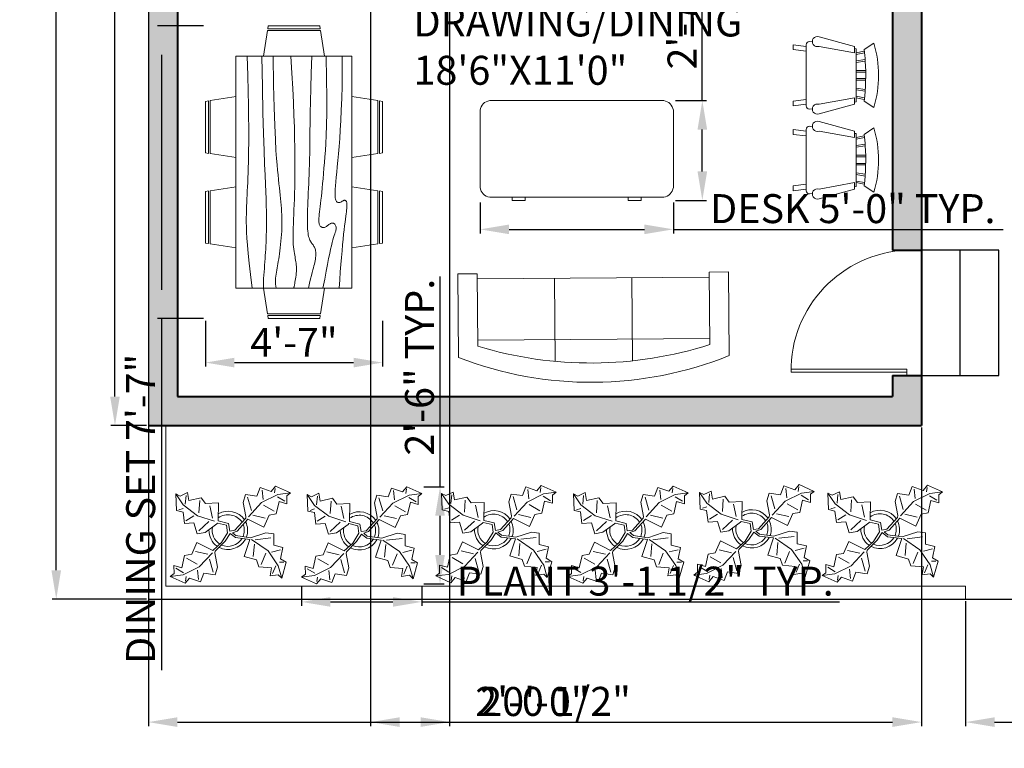
# Model space of a CAD drawing. Units: inches. Extents: x 1967493 to 1968177, y 907234 to 908105.
# Tile 1 of 5: x 1967549 to 1967854, y 907234 to 907460. Entities that reach past the tile are written whole.
import ezdxf

# ---------------------------------------------------------------- set-up
doc = ezdxf.new("R2010")
doc.units = ezdxf.units.IN
for name, color, linetype, lineweight in [('A-ANNO-DIMS', 2, 'Continuous', 18), ('A-AREA-IDEN', 7, 'Continuous', 25), ('A-DOOR', 3, 'Continuous', 20), ('A-FLOR-STRS', 7, 'Continuous', 25), ('A-FURN', 8, 'Continuous', 18), ('A-WALL', 7, 'Continuous', 40), ('C-PROP', 7, 'Continuous', 25), ('L-PLNT', 94, 'Continuous', 18)]:
    doc.layers.add(name, color=color, linetype=linetype, lineweight=lineweight)
doc.layers.add('A-WALL-PATT', color=18, linetype='Continuous', lineweight=13, true_color=0x000000)
doc.styles.get("Standard").update_dxf_attribs({"font": 'arial.ttf'})
doc.dimstyles.new('ISO-25', dxfattribs={"dimtxt": 9, "dimasz": 9, "dimexe": 1.25, "dimexo": 0.625, "dimtad": 1, "dimdec": 1, "dimrnd": 9, "dimlunit": 3, "dimtxsty": 'Standard', "dimcen": 2.5, "dimadec": 0, "dimazin": 0, "dimtfac": 1, "dimtdec": 1, "dimtmove": 0, "dimatfit": 3, "dimfxl": 1, "dimarcsym": 0})

# ---------------------------------------------------------------- blocks, each defined once
blk = doc.blocks.new('Plant - Rubber or Philodendron')
for p, q in [((8.8871, 10.7908), (9.9809, 13.4933)), ((9.9809, 13.4933), (13.3837, 12.301)), ((10.5828, 12.6946), (10.8893, 9.7953)), ((13.3837, 12.301), (14.68, 13.9039)), ((14.5816, 13.2037), (14.3848, 11.8033)), ((14.68, 13.9039), (19.3848, 11.8146)), ((-16.2005, 11.4774), (-13.9899, 8.1064)), ((-16.2005, 11.4774), (-14.8639, 10.7964)), ((-16.0159, 6.3329), (-16.2005, 11.4774)), ((-14.8639, 10.7964), (-12.6195, 11.8975)), ((-13.3174, 8.325), (-13.0735, 11.0065)), ((-12.6195, 11.8975), (-12.1909, 9.4345)), ((-12.1909, 9.4345), (-8.3829, 10.3)), ((-8.8369, 9.409), (-9.0894, 5.6095)), ((-8.3829, 10.3), (-7.0549, 8.501)), ((4.6914, 8.8812), (5.3859, 11.2828)), ((5.3859, 11.2828), (8.8871, 10.7908)), ((5.9878, 10.4842), (7.1971, 6.3869)), ((15.3859, 11.3055), (10.3916, 8.7942)), ((15.2875, 10.6053), (17.5907, 9.2105)), ((19.3848, 11.8146), (15.3859, 11.3055)), ((19.3848, 11.8146), (18.1868, 10.9119)), ((18.1868, 10.9119), (18.1925, 8.4119)), ((-14.0069, 5.8704), (-16.0159, 6.3329)), ((-15.3434, 6.5514), (-13.9984, 6.9884)), ((-13.9899, 8.1064), (-9.5434, 4.7185)), ((-7.0549, 8.501), (-3.0284, 8.6941)), ((-4.8529, 4.012), (-5.7184, 7.82)), ((-3.0284, 8.6941), (-3.0709, 3.1041)), ((4.6914, 8.8812), (5.5014, 4.4831)), ((10.3916, 8.7942), (6.2847, 4.4028)), ((14.2977, 6.1031), (10.9934, 7.9956)), ((15.7909, 9.1065), (14.8995, 5.3044)), ((18.1925, 8.4119), (15.7909, 9.1065)), ((-13.5868, 2.2894), (-14.0069, 5.8704)), ((-13.1329, 3.1804), (-10.6614, 4.727)), ((-9.5434, 4.7185), (-4.1917, 2.9888)), ((-3.0709, 3.1041), (0.0797, 2.3163)), ((2.1141, 0.2298), (5.4346, 3.9146)), ((6.1032, 3.6844), (2.8262, -0.031)), ((5.4346, 3.9146), (5.5014, 4.4831)), ((11.1089, 1.1958), (6.1032, 3.6844)), ((7.7005, 4.8881), (11.5025, 3.9967)), ((12.7005, 4.8994), (11.1089, 1.1958)), ((14.8995, 5.3044), (12.7005, 4.8994)), ((-10.6784, 2.491), (-13.5868, 2.2894)), ((-9.5858, -0.8715), (-10.6784, 2.491)), ((-9.1318, 0.0195), (-5.9793, 2.9025)), ((-7.1228, -0.443), (-3.5248, 2.2131)), ((-3.5248, 2.2131), (-3.3011, 2.4355)), ((-3.3011, 2.4355), (-0.5306, 1.7947)), ((-0.5306, 1.7947), (-0.2255, -0.5527)), ((-0.5306, 1.7947), (-0.5306, 1.7947)), ((0.0797, 2.3163), (0.4866, -0.031)), ((0.4866, -0.031), (2.1141, 0.2298)), ((-7.1228, -0.443), (-9.5858, -0.8715)), ((-2.019, -3.6148), (-0.2255, -0.5527)), ((-0.9375, -3.1608), (0.5883, -0.8135)), ((0.5883, -0.8135), (2.2447, -2.0916)), ((2.8262, -0.031), (1.3003, -0.5527)), ((1.3003, -0.5527), (2.4193, -1.4655)), ((2.2447, -2.0916), (6.7108, -2.6626)), ((2.4193, -1.4655), (6.895, -2.1175)), ((4.943, -7.9659), (6.7108, -2.6626)), ((11.6605, -0.5413), (6.895, -2.1175)), ((12.3677, -6.1981), (7.219, -2.6772)), ((8.3544, -2.7453), (13.1973, -2.1704)), ((11.6605, -0.5413), (14.1354, -0.8948)), ((14.1354, -0.8948), (14.1354, -4.4304)), ((-11.3237, -7.2629), (-9.7321, -3.5593)), ((-9.7321, -3.5593), (-4.7264, -6.0479)), ((-2.019, -3.6148), (-4.7264, -6.0479)), ((-4.0579, -6.2781), (-0.9375, -3.1608)), ((8.125, -4.0768), (7.7715, -7.9659)), ((16.2567, -5.8446), (13.4283, -6.5517)), ((14.1354, -4.4304), (16.9638, -5.1375)), ((16.9638, -5.1375), (16.2567, -8.673)), ((-14.4141, -11.4699), (-13.5228, -7.6679)), ((-13.5228, -7.6679), (-11.3237, -7.2629)), ((-12.921, -8.4665), (-9.6166, -10.359)), ((-6.3237, -7.2516), (-10.1257, -6.3602)), ((-9.0148, -11.1577), (-4.9047, -6.8122)), ((-4.611, -12.8477), (-5.8203, -8.7504)), ((-4.1246, -6.8466), (-4.0579, -6.2781)), ((-3.3146, -11.2447), (-4.1246, -6.8466)), ((8.8321, -9.0266), (4.943, -7.9659)), ((9.5392, -11.1479), (8.8321, -9.0266)), ((10.2463, -10.4408), (11.6605, -6.9053)), ((15.5496, -10.7943), (12.3677, -6.1981)), ((16.2567, -8.673), (18.0245, -9.7337)), ((-16.8157, -10.7754), (-14.4141, -11.4699)), ((-16.8101, -13.2754), (-16.8157, -10.7754)), ((-13.9107, -12.9688), (-16.2139, -11.574)), ((-14.0091, -13.669), (-9.0148, -11.1577)), ((-9.206, -15.0581), (-9.5126, -12.1588)), ((-3.3146, -11.2447), (-4.0092, -13.6463)), ((13.4283, -11.5015), (9.5392, -11.1479)), ((13.0748, -13.9763), (13.4283, -11.5015)), ((14.8425, -10.7943), (13.7819, -13.2692)), ((16.6103, -14.6834), (15.5496, -10.7943)), ((17.3174, -9.7337), (15.9032, -9.7337)), ((18.0245, -9.7337), (16.6103, -14.6834)), ((-18.008, -14.1781), (-16.8101, -13.2754)), ((-18.008, -14.1781), (-14.0091, -13.669)), ((-13.3032, -16.2674), (-18.008, -14.1781)), ((-12.0069, -14.6645), (-13.3032, -16.2674)), ((-13.2048, -15.5672), (-13.008, -14.1668)), ((-8.6042, -15.8568), (-12.0069, -14.6645)), ((-7.5103, -13.1543), (-8.6042, -15.8568)), ((-4.0092, -13.6463), (-7.5103, -13.1543)), ((15.5496, -13.6228), (13.0748, -13.9763)), ((16.6103, -14.6834), (15.5496, -13.6228))]:
    blk.add_line(p, q)
for centre, radius, start, end in [((0, 0), 6.1275, 34.37569, 120.1028), ((-0.0601, -0.2075), 5.2461, 33.82192, 124.9414), ((0.0308, 0.1664), 6, 178.6147, 235.1169), ((0.0308, 0.1664), 5, 168.1647, 238.6725), ((-0.2664, 0.1682), 5.2775, 338.4094, 20.03007), ((-0.098, 0.1364), 6.1288, 341.2017, 26.09184), ((-0.0234, 0.3825), 6.1492, 242.5812, 331.2714), ((-0.1102, 0.4886), 5.2883, 247.3711, 327.472)]:
    blk.add_arc(centre, radius, start, end)
blk = doc.blocks.new('Dining Set - 36 x 72 in.')
for p, q in [((-22.2343, 26.00059), (-23.4847, 17.99762)), ((-22.2304, 26), (-5.7608, 26)), ((-22, 27.5), (-22.1562, 26.50042)), ((-5.8416, 26.5), (-22.1534, 26.5)), ((-22, 27.5), (-6, 27.5)), ((-5.8437, 26.49966), (-6, 27.5)), ((-4.5152, 17.99762), (-5.7655, 25.99926)), ((5.7657, 26.00059), (4.5153, 17.99762)), ((5.7696, 26), (22.2392, 26)), ((6, 27.5), (5.8438, 26.50042)), ((22.1584, 26.5), (5.8466, 26.5)), ((6, 27.5), (22, 27.5)), ((22.1563, 26.49966), (22, 27.5)), ((23.4848, 17.99762), (22.2345, 25.99926)), ((36, 18), (-36, 18)), ((-36, 18), (-36, -18)), ((36, -18), (36, 18)), ((-44.0006, 8.23428), (-35.9976, 9.48474)), ((44.0006, 8.23428), (35.9976, 9.48474)), ((-45.5, 8), (-44.5004, 8.15617)), ((-45.5, 8), (-45.5, -8)), ((-44.5, -8.15843), (-44.5, 8.15338)), ((-44, 8.23041), (-44, -8.23915)), ((44, 8.23041), (44, -8.23915)), ((44.5, -8.15843), (44.5, 8.15338)), ((45.5, 8), (44.5005, 8.15617)), ((45.5, 8), (45.5, -8)), ((-44.4997, -8.15631), (-45.5, -8)), ((-35.9976, -9.48476), (-43.9993, -8.2345)), ((35.9976, -9.48476), (43.9993, -8.2345)), ((44.4997, -8.15631), (45.5, -8)), ((-36, -18), (36, -18)), ((-22.2343, -26.0006), (-23.4847, -17.99762)), ((-4.5152, -17.99762), (-5.7655, -25.99928)), ((5.7657, -26.0006), (4.5153, -17.99762)), ((23.4848, -17.99762), (22.2345, -25.99928)), ((-22.2304, -26), (-5.7608, -26)), ((-22, -27.5), (-22.1562, -26.50044)), ((-5.8416, -26.5), (-22.1534, -26.5)), ((-22, -27.5), (-6, -27.5)), ((-5.8437, -26.49967), (-6, -27.5)), ((5.7696, -26), (22.2392, -26)), ((6, -27.5), (5.8438, -26.50044)), ((22.1584, -26.5), (5.8466, -26.5)), ((6, -27.5), (22, -27.5)), ((22.1563, -26.49967), (22, -27.5))]:
    blk.add_line(p, q)
for points in [[(-36, 15), (-31.1772, 14.97754), (-26.8079, 14.91406), (-22.8538, 14.81543), (-19.276, 14.6875), (-16.0362, 14.53613), (-13.0957, 14.36718), (-10.4159, 14.18652), (-7.9583, 14), (-5.6904, 13.81315), (-3.6035, 13.63021), (-1.6954, 13.45508), (0.0365, 13.29166), (1.5945, 13.14388), (2.9811, 13.01562), (4.1988, 12.9108), (5.25, 12.83333), (6.1393, 12.78613), (6.8802, 12.76823), (7.4883, 12.77767), (7.9792, 12.8125), (8.3685, 12.87077), (8.6719, 12.95052), (8.9049, 13.0498), (9.0833, 13.16666), (9.2205, 13.29899), (9.3216, 13.44401), (9.3895, 13.59879), (9.4271, 13.76041), (9.4373, 13.92594), (9.4232, 14.09245), (9.3875, 14.257), (9.3333, 14.41666), (9.2638, 14.56917), (9.1836, 14.71484), (9.0975, 14.85465), (9.0104, 14.98958), (8.9272, 15.1206), (8.8529, 15.2487), (8.7922, 15.37483), (8.75, 15.5), (8.7305, 15.62467), (8.7344, 15.74739), (8.7617, 15.86621), (8.8125, 15.97916), (8.8867, 16.08431), (8.9844, 16.17968), (9.1055, 16.26334), (9.25, 16.33333), (9.4189, 16.38802), (9.6172, 16.42708), (9.8506, 16.45052), (10.125, 16.45833), (10.4463, 16.45052), (10.8203, 16.42708), (11.2529, 16.38802), (11.75, 16.33333), (12.3184, 16.26318), (12.9694, 16.17838), (13.7151, 16.07991), (14.5677, 15.96875), (15.5395, 15.84586), (16.6426, 15.71224), (17.8893, 15.56884), (19.2917, 15.41666), (20.859, 15.25667), (22.5879, 15.08984), (24.4721, 14.91715), (26.5052, 14.73958), (28.6809, 14.5581), (30.9929, 14.3737), (33.4347, 14.18733), (36, 14)], [(-36, 10), (-28.9766, 10.14274), (-23.1725, 10.20442), (-18.4241, 10.19775), (-14.5677, 10.13541), (-11.4399, 10.03011), (-8.877, 9.89453), (-6.7154, 9.74137), (-4.7917, 9.58333), (-2.9698, 9.43082), (-1.2246, 9.28515), (0.4415, 9.14534), (2.026, 9.01041), (3.5266, 8.87939), (4.9408, 8.7513), (6.266, 8.62516), (7.5, 8.5), (8.6411, 8.37549), (9.6914, 8.2539), (10.6538, 8.13818), (11.5312, 8.03125), (12.3267, 7.93603), (13.043, 7.85547), (13.6831, 7.79248), (14.25, 7.75), (14.7471, 7.7303), (15.1797, 7.73307), (15.5537, 7.75732), (15.875, 7.80208), (16.1494, 7.86637), (16.3828, 7.94922), (16.5811, 8.04964), (16.75, 8.16666), (16.8944, 8.29915), (17.0143, 8.44531), (17.1089, 8.60319), (17.1771, 8.77083), (17.218, 8.94629), (17.2305, 9.1276), (17.2137, 9.31282), (17.1667, 9.5), (17.0895, 9.6875), (16.987, 9.875), (16.8649, 10.0625), (16.7292, 10.25), (16.5856, 10.4375), (16.4401, 10.625), (16.2985, 10.8125), (16.1667, 11), (16.05, 11.18733), (15.9518, 11.3737), (15.8752, 11.5581), (15.8229, 11.73958), (15.798, 11.91715), (15.8034, 12.08984), (15.842, 12.25667), (15.9167, 12.41666), (16.0295, 12.56836), (16.1784, 12.70833), (16.3605, 12.83268), (16.5729, 12.9375), (16.8127, 13.01888), (17.0768, 13.07291), (17.3625, 13.0957), (17.6667, 13.08333), (17.9894, 13.03312), (18.3418, 12.94726), (18.7382, 12.82918), (19.1927, 12.68229), (19.7195, 12.51001), (20.3327, 12.31575), (21.0465, 12.10294), (21.875, 11.875), (22.8357, 11.63354), (23.959, 11.37304), (25.2786, 11.08618), (26.8282, 10.76562), (28.6414, 10.40405), (30.752, 9.99414), (33.1936, 9.52856), (36, 9)], [(-36, 5.5), (-30.7157, 5.3348), (-26.069, 5.20963), (-21.9946, 5.11767), (-18.4271, 5.05208), (-15.3009, 5.00602), (-12.5508, 4.97265), (-10.1112, 4.94515), (-7.9167, 4.91666), (-5.909, 4.88167), (-4.0586, 4.83984), (-2.3429, 4.79215), (-0.7396, 4.73958), (0.7739, 4.6831), (2.22, 4.6237), (3.6213, 4.56233), (5, 4.5), (6.373, 4.43782), (7.7344, 4.3776), (9.0723, 4.32129), (10.375, 4.27083), (11.6309, 4.22819), (12.8281, 4.19531), (13.9551, 4.17415), (15, 4.16666), (15.954, 4.17448), (16.819, 4.19791), (17.6001, 4.23698), (18.3021, 4.29166), (18.9299, 4.36198), (19.4883, 4.44791), (19.9823, 4.54948), (20.4167, 4.66666), (20.7969, 4.79899), (21.1302, 4.94401), (21.4245, 5.09879), (21.6875, 5.26041), (21.9271, 5.42594), (22.1511, 5.59245), (22.3672, 5.757), (22.5834, 5.91666), (22.8065, 6.06868), (23.0404, 6.21093), (23.2879, 6.34147), (23.5521, 6.45833), (23.8358, 6.55957), (24.142, 6.64323), (24.4735, 6.70735), (24.8334, 6.75), (25.2235, 6.76969), (25.642, 6.76692), (26.0858, 6.74267), (26.5521, 6.69791), (27.0379, 6.63362), (27.5404, 6.55078), (28.0565, 6.45036), (28.5834, 6.33333), (29.1242, 6.19987), (29.7071, 6.04687), (30.3661, 5.87044), (31.1354, 5.66666), (32.0493, 5.43164), (33.142, 5.16146), (34.4475, 4.85221), (36, 4.5)], [(-36, -1), (-30.7915, -0.6591), (-26.0195, -0.38216), (-21.6519, -0.16284), (-17.6563, 0.00521), (-14.0005, 0.12833), (-10.6523, 0.21289), (-7.5796, 0.26522), (-4.75, 0.29166), (-2.134, 0.29793), (0.2878, 0.28711), (2.5317, 0.26163), (4.6146, 0.22396), (6.5529, 0.17651), (8.3633, 0.12174), (10.0623, 0.06209), (11.6667, 0), (13.1899, -0.06201), (14.6341, -0.1211), (15.9982, -0.17432), (17.2813, -0.21875), (18.4823, -0.25147), (19.6003, -0.26953), (20.6343, -0.27002), (21.5834, -0.25), (22.4481, -0.20768), (23.2357, -0.14584), (23.9549, -0.06836), (24.6146, 0.02083), (25.2235, 0.11784), (25.7904, 0.21875), (26.3241, 0.31966), (26.8334, 0.41666), (27.3265, 0.50618), (27.8099, 0.58593), (28.2894, 0.65397), (28.7709, 0.70833), (29.2601, 0.74707), (29.763, 0.76823), (30.2855, 0.76985), (30.8334, 0.75), (31.4088, 0.70784), (31.9994, 0.64713), (32.589, 0.57275), (33.1615, 0.48958), (33.7008, 0.4025), (34.1908, 0.3164), (34.6153, 0.23616), (34.9584, 0.16666), (35.2099, 0.11165), (35.3848, 0.07031), (35.504, 0.04069), (35.5886, 0.02083), (35.6594, 0.00879), (35.7377, 0.0026), (35.8442, 0.00032), (36, 0)], [(-36, -6.5), (-27.1843, -6.31267), (-20.084, -6.1263), (-14.469, -5.9419), (-10.1094, -5.76042), (-6.7752, -5.58285), (-4.2363, -5.41016), (-2.2629, -5.24333), (-0.625, -5.08334), (0.8708, -4.93099), (2.2715, -4.78646), (3.5872, -4.64974), (4.8281, -4.52084), (6.0046, -4.39974), (7.127, -4.28646), (8.2053, -4.18099), (9.25, -4.08334), (10.2705, -3.99382), (11.2734, -3.91407), (12.2647, -3.84603), (13.25, -3.79167), (14.2354, -3.75293), (15.2266, -3.73177), (16.2295, -3.73015), (17.25, -3.75), (18.2912, -3.79248), (19.3451, -3.85547), (20.4009, -3.93604), (21.4479, -4.03125), (22.4754, -4.13819), (23.4727, -4.25391), (24.4289, -4.37549), (25.3334, -4.5), (26.1785, -4.62492), (26.9694, -4.74935), (27.7145, -4.87281), (28.4219, -4.99479), (29.1, -5.11483), (29.7572, -5.23242), (30.4016, -5.34709), (31.0417, -5.45834), (31.6837, -5.56437), (32.3262, -5.65821), (32.9658, -5.73153), (33.599, -5.77604), (34.2224, -5.78345), (34.8327, -5.74545), (35.4264, -5.65373), (36, -5.5)], [(-36, -10), (-26.4022, -9.81299), (-18.4675, -9.62891), (-11.9839, -9.45069), (-6.7396, -9.28125), (-2.5226, -9.12354), (0.8789, -8.98047), (3.6769, -8.85498), (6.0833, -8.75), (8.2767, -8.66765), (10.3021, -8.60677), (12.1712, -8.56543), (13.8958, -8.54167), (15.4876, -8.53353), (16.9583, -8.53907), (18.3197, -8.55632), (19.5834, -8.58334), (20.7616, -8.61841), (21.8685, -8.66081), (22.9188, -8.71004), (23.9271, -8.76563), (24.9081, -8.82707), (25.8763, -8.89388), (26.8465, -8.96558), (27.8334, -9.04167), (28.8474, -9.12118), (29.8828, -9.20117), (30.93, -9.27824), (31.9792, -9.34896), (33.0205, -9.40991), (34.0443, -9.45768), (35.0407, -9.48885), (36, -9.5)], [(-36, -14.5), (-30.0881, -14.33513), (-25.0332, -14.21224), (-20.7312, -14.12647), (-17.0781, -14.07292), (-13.97, -14.04671), (-11.3027, -14.04297), (-8.9724, -14.05681), (-6.875, -14.08334), (-4.9224, -14.11833), (-3.0905, -14.16016), (-1.3709, -14.20785), (0.2448, -14.26042), (1.7647, -14.3169), (3.1973, -14.3763), (4.5507, -14.43767), (5.8333, -14.5), (7.0554, -14.5621), (8.235, -14.62175), (9.3922, -14.67652), (10.5469, -14.72396), (11.7192, -14.76164), (12.929, -14.78711), (14.1965, -14.79794), (15.5417, -14.79167), (16.9933, -14.76424), (18.6152, -14.70508), (20.4804, -14.60197), (22.6615, -14.44271), (25.2312, -14.21509), (28.2624, -13.9069), (31.8277, -13.50594), (36, -13)]]:
    blk.add_lwpolyline(points)
blk = doc.blocks.new('Sofa - Roundback 7 ft.')
for p, q in [((-12.00002, -32.4421), (-12.00003, -6.5971)), ((11.99997, -32.4421), (11.99998, -6.5971)), ((-36.000027, -34), (-36.000027, -11.4696)), ((35.99998, -34), (35.99998, -11.4696)), ((-35.999844, -13.3819), (35.9998, -13.3819)), ((-36.000027, -32.4421), (35.99998, -32.4421))]:
    blk.add_line(p, q)
for points in [[(-36.000027, -34), (-42.000027, -34), (-42.000027, -8)], [(41.99998, -8), (41.99998, -34), (35.99998, -34)]]:
    blk.add_lwpolyline(points)
for centre, radius, start, end in [((0, -114.25), 114.25, 68.43141, 111.5686), ((-0.00001, -127.1968), 121.1968, 72.72033, 107.2797)]:
    blk.add_arc(centre, radius, start, end)
blk = doc.blocks.new('Desk - 30 x 60 in.')
for p, q in [((-26.999995, 0), (26.999995, 0)), ((-29.999995, -27), (-29.999995, -3)), ((29.999995, -3), (29.999995, -27)), ((26.999995, -30), (-26.999995, -30)), ((-20.000005, -30), (-20.000005, -31)), ((-16.000005, -31), (-16.000005, -30)), ((15.999995, -31), (15.999995, -30)), ((19.999995, -30), (19.999995, -31)), ((-20.000005, -31), (-16.000005, -31)), ((19.999995, -31), (15.999995, -31))]:
    blk.add_line(p, q)
for centre, start, end in [((-26.499995, -3.5), 98.1301, 171.8699), ((26.499995, -3.5), 8.130102, 81.8699), ((-26.499995, -26.5), 188.1301, 261.8699), ((26.499995, -26.5), 278.1301, 351.8699)]:
    blk.add_arc(centre, 3.535534, start, end)
blk = doc.blocks.new('Chair - Rocking')
for p, q in [((-8, -4.5), (-10, -1.5)), ((8, -4.5), (10, -1.5)), ((-7.5, -4.5), (-7, -7)), ((-6.5, -7), (-7.02225, -4.43)), ((-4.5, -7), (-4.96674, -4.19951)), ((-4, -7), (-4.40532, -4.16272)), ((-1.5, -4.05012), (-1.5, -7)), ((-1, -7), (-1, -4.05012)), ((1, -7), (1, -4.04655)), ((1.5, -4.05012), (1.5, -7)), ((4, -7), (4.40187, -4.18694)), ((4.5, -7), (4.96761, -4.19437)), ((6.5, -7), (7, -4.4057)), ((7.5, -4.5), (7, -7)), ((-9, -7.5), (-12, -18.49999)), ((-7, -7.5), (-9, -7.5)), ((-9, -18.49999), (-7, -7.5)), ((-8.23428, -6.99939), (-8.3093, -7.47958)), ((-8.23041, -7), (8.23915, -7)), ((7, -7.5), (9, -7.5)), ((9, -18.49999), (7, -7.5)), ((8.31071, -7.48854), (8.23449, -7.00073)), ((9, -7.5), (12, -18.49999)), ((-10.36644, -20.64523), (-10.5, -21.49999)), ((10.5, -21.49999), (10.3575, -20.58798)), ((-9, -22.49999), (-9.5, -26.49999)), ((0, -22.49999), (-9.5, -22.49999)), ((-8, -26.49999), (-7.5, -22.49999)), ((0, -22.49999), (9.5, -22.49999)), ((8, -26.49999), (7.5, -22.49999)), ((9, -22.49999), (9.5, -26.49999)), ((-9.5, -26.49999), (-8, -26.49999)), ((9.5, -26.49999), (8, -26.49999))]:
    blk.add_line(p, q)
for centre, radius, start, end in [((0, -34.08333), 34.08333, 72.93847, 107.0615), ((0, -68.25004), 64.25, 93.92211, 97.15267), ((0, -68.25004), 64.25, 82.84733, 93.92211), ((-10.5, -18.99999), 1.58114, 161.5651, 18.43495), ((10.5, -18.99999), 1.58114, 161.5651, 18.43495), ((-9.5, -21.49999), 1, 180, 270), ((9.5, -21.49999), 1, 270, 0)]:
    blk.add_arc(centre, radius, start, end)
blk = doc.blocks.new('*D12')
at = {"layer": 'A-ANNO-DIMS', "color": 0, "lineweight": -2, "transparency": 16777216}
for p, q in [((1967588.15, 908000.17), (1967558.93, 908000.17)), ((1967560.18, 907289.17), (1967560.18, 907991.17)), ((1967588.15, 907280.17), (1967558.93, 907280.17))]:
    blk.add_line(p, q, dxfattribs=at)
at = {"layer": 'A-ANNO-DIMS', "color": 0, "transparency": 16777216}
for points in [[(1967558.68, 907991.17), (1967561.68, 907991.17), (1967560.18, 908000.17)], [(1967558.68, 907289.17), (1967561.68, 907289.17), (1967560.18, 907280.17)]]:
    blk.add_solid(points, dxfattribs=at)
at = {"layer": 'Defpoints', "color": 0, "transparency": 16777216}
for p in [(1967560.18, 908000.17), (1967588.78, 908000.17), (1967588.78, 907280.17)]:
    blk.add_point(p, dxfattribs=at)
at = {"layer": 'A-ANNO-DIMS', "color": 0, "transparency": 16777216, "insert": (1967554.96, 907640.17), "char_height": 9, "attachment_point": 5, "rotation": 90}
blk.add_mtext("60'", dxfattribs=at)
blk = doc.blocks.new('*D13')
at = {"layer": 'A-ANNO-DIMS', "color": 0, "lineweight": -2, "transparency": 16777216}
for p, q in [((1967588.15, 908000.17), (1967577.16, 908000.17)), ((1967578.41, 907343.17), (1967578.41, 907991.17)), ((1967588.15, 907334.17), (1967577.16, 907334.17))]:
    blk.add_line(p, q, dxfattribs=at)
at = {"layer": 'A-ANNO-DIMS', "color": 0, "transparency": 16777216}
for points in [[(1967576.91, 907991.17), (1967579.91, 907991.17), (1967578.41, 908000.17)], [(1967576.91, 907343.17), (1967579.91, 907343.17), (1967578.41, 907334.17)]]:
    blk.add_solid(points, dxfattribs=at)
at = {"layer": 'Defpoints', "color": 0, "transparency": 16777216}
for p in [(1967578.41, 908000.17), (1967588.78, 908000.17), (1967588.78, 907334.17)]:
    blk.add_point(p, dxfattribs=at)
at = {"layer": 'A-ANNO-DIMS', "color": 0, "transparency": 16777216, "insert": (1967573.19, 907667.17), "char_height": 9, "attachment_point": 5, "rotation": 90}
blk.add_mtext('55\'-6"', dxfattribs=at)
blk = doc.blocks.new('*D20')
at = {"layer": 'A-ANNO-DIMS', "color": 0, "lineweight": -2, "transparency": 16777216}
for p, q in [((1967636.31, 907284.35), (1967636.31, 907278.11)), ((1967673.71, 907284.35), (1967673.71, 907278.11)), ((1967645.31, 907279.36), (1967664.71, 907279.36)), ((1967673.71, 907279.36), (1967803.36, 907279.36))]:
    blk.add_line(p, q, dxfattribs=at)
at = {"layer": 'A-ANNO-DIMS', "color": 0, "transparency": 16777216}
for points in [[(1967645.31, 907280.86), (1967645.31, 907277.86), (1967636.31, 907279.36)], [(1967664.71, 907280.86), (1967664.71, 907277.86), (1967673.71, 907279.36)]]:
    blk.add_solid(points, dxfattribs=at)
at = {"layer": 'Defpoints', "color": 0, "transparency": 16777216}
for p in [(1967636.31, 907284.97), (1967673.71, 907284.97), (1967673.71, 907279.36)]:
    blk.add_point(p, dxfattribs=at)
at = {"layer": 'A-ANNO-DIMS', "color": 0, "transparency": 16777216, "insert": (1967743.03, 907284.65), "char_height": 9, "attachment_point": 5}
blk.add_mtext('PLANT 3\'-1 1/2" TYP.', dxfattribs=at)
blk = doc.blocks.new('*D21')
at = {"layer": 'A-ANNO-DIMS', "color": 0, "lineweight": -2, "transparency": 16777216}
for p, q in [((1967679.32, 907315.14), (1967679.32, 907380.41)), ((1967674.33, 907315.14), (1967680.57, 907315.14)), ((1967679.32, 907293.97), (1967679.32, 907306.14)), ((1967674.33, 907284.97), (1967680.57, 907284.97))]:
    blk.add_line(p, q, dxfattribs=at)
at = {"layer": 'A-ANNO-DIMS', "color": 0, "transparency": 16777216}
for points in [[(1967677.82, 907306.14), (1967680.82, 907306.14), (1967679.32, 907315.14)], [(1967677.82, 907293.97), (1967680.82, 907293.97), (1967679.32, 907284.97)]]:
    blk.add_solid(points, dxfattribs=at)
at = {"layer": 'Defpoints', "color": 0, "transparency": 16777216}
for p in [(1967673.71, 907315.14), (1967679.32, 907315.14), (1967673.71, 907284.97)]:
    blk.add_point(p, dxfattribs=at)
at = {"layer": 'A-ANNO-DIMS', "color": 0, "transparency": 16777216, "insert": (1967674.1, 907352.28), "char_height": 9, "attachment_point": 5, "rotation": 90}
blk.add_mtext('2\'-6" TYP.', dxfattribs=at)
blk = doc.blocks.new('*D32')
at = {"layer": 'A-ANNO-DIMS', "color": 0, "lineweight": -2, "transparency": 16777216}
for p, q in [((1967691.75, 907403.47), (1967691.75, 907393.85)), ((1967751.75, 907403.47), (1967751.75, 907393.85)), ((1967700.75, 907395.1), (1967742.75, 907395.1)), ((1967751.75, 907395.1), (1967854.15, 907395.1))]:
    blk.add_line(p, q, dxfattribs=at)
at = {"layer": 'A-ANNO-DIMS', "color": 0, "transparency": 16777216}
for points in [[(1967700.75, 907396.6), (1967700.75, 907393.6), (1967691.75, 907395.1)], [(1967742.75, 907396.6), (1967742.75, 907393.6), (1967751.75, 907395.1)]]:
    blk.add_solid(points, dxfattribs=at)
at = {"layer": 'Defpoints', "color": 0, "transparency": 16777216}
for p in [(1967691.75, 907404.1), (1967751.75, 907404.1), (1967751.75, 907395.1)]:
    blk.add_point(p, dxfattribs=at)
at = {"layer": 'A-ANNO-DIMS', "color": 0, "transparency": 16777216, "insert": (1967807.45, 907400.37), "char_height": 9, "attachment_point": 5}
blk.add_mtext('DESK 5\'-0" TYP.', dxfattribs=at)
blk = doc.blocks.new('*D33')
at = {"layer": 'A-ANNO-DIMS', "color": 0, "lineweight": -2, "transparency": 16777216}
for p, q in [((1967760.75, 907435.1), (1967760.75, 907500.36)), ((1967752.38, 907435.1), (1967762, 907435.1)), ((1967760.75, 907413.1), (1967760.75, 907426.1)), ((1967752.38, 907404.1), (1967762, 907404.1))]:
    blk.add_line(p, q, dxfattribs=at)
at = {"layer": 'A-ANNO-DIMS', "color": 0, "transparency": 16777216}
for points in [[(1967759.25, 907426.1), (1967762.25, 907426.1), (1967760.75, 907435.1)], [(1967759.25, 907413.1), (1967762.25, 907413.1), (1967760.75, 907404.1)]]:
    blk.add_solid(points, dxfattribs=at)
at = {"layer": 'Defpoints', "color": 0, "transparency": 16777216}
for p in [(1967751.75, 907435.1), (1967760.75, 907435.1), (1967751.75, 907404.1)]:
    blk.add_point(p, dxfattribs=at)
at = {"layer": 'A-ANNO-DIMS', "color": 0, "transparency": 16777216, "insert": (1967755.61, 907472.23), "char_height": 9, "attachment_point": 5, "rotation": 90}
blk.add_mtext('2\'-7" TYP.', dxfattribs=at)
blk = doc.blocks.new('*D38')
at = {"layer": 'A-ANNO-DIMS', "color": 0, "lineweight": -2, "transparency": 16777216}
for p, q in [((1967605.85, 907458.36), (1967591.58, 907458.36)), ((1967592.83, 907449.36), (1967592.83, 907376.36)), ((1967605.85, 907367.36), (1967591.58, 907367.36)), ((1967592.83, 907367.36), (1967592.83, 907258.19))]:
    blk.add_line(p, q, dxfattribs=at)
at = {"layer": 'A-ANNO-DIMS', "color": 0, "transparency": 16777216}
for points in [[(1967591.33, 907449.36), (1967594.33, 907449.36), (1967592.83, 907458.36)], [(1967591.33, 907376.36), (1967594.33, 907376.36), (1967592.83, 907367.36)]]:
    blk.add_solid(points, dxfattribs=at)
at = {"layer": 'Defpoints', "color": 0, "transparency": 16777216}
for p in [(1967606.48, 907458.36), (1967592.83, 907367.36), (1967606.48, 907367.36)]:
    blk.add_point(p, dxfattribs=at)
at = {"layer": 'A-ANNO-DIMS', "color": 0, "transparency": 16777216, "insert": (1967587.55, 907308.27), "char_height": 9, "attachment_point": 5, "rotation": 90}
blk.add_mtext('DINING SET 7\'-7"', dxfattribs=at)
blk = doc.blocks.new('*D39')
at = {"layer": 'A-ANNO-DIMS', "color": 0, "lineweight": -2, "transparency": 16777216}
for p, q in [((1967606.48, 907366.73), (1967606.48, 907352.46)), ((1967661.48, 907366.73), (1967661.48, 907352.46)), ((1967615.48, 907353.71), (1967652.48, 907353.71))]:
    blk.add_line(p, q, dxfattribs=at)
at = {"layer": 'A-ANNO-DIMS', "color": 0, "transparency": 16777216}
for points in [[(1967615.48, 907355.21), (1967615.48, 907352.21), (1967606.48, 907353.71)], [(1967652.48, 907355.21), (1967652.48, 907352.21), (1967661.48, 907353.71)]]:
    blk.add_solid(points, dxfattribs=at)
at = {"layer": 'Defpoints', "color": 0, "transparency": 16777216}
for p in [(1967606.48, 907367.36), (1967661.48, 907367.36), (1967661.48, 907353.71)]:
    blk.add_point(p, dxfattribs=at)
at = {"layer": 'A-ANNO-DIMS', "color": 0, "transparency": 16777216, "insert": (1967633.98, 907358.83), "char_height": 9, "attachment_point": 5}
blk.add_mtext('4\'-7"', dxfattribs=at)
blk = doc.blocks.new('*D46')
at = {"layer": 'A-ANNO-DIMS', "color": 0, "lineweight": -2, "transparency": 16777216}
for p, q in [((1967842.47, 907279.54), (1967842.47, 907240.77)), ((1968059.78, 907279.54), (1968059.78, 907240.77)), ((1967851.47, 907242.02), (1968050.78, 907242.02))]:
    blk.add_line(p, q, dxfattribs=at)
at = {"layer": 'A-ANNO-DIMS', "color": 0, "transparency": 16777216}
for points in [[(1967851.47, 907243.52), (1967851.47, 907240.52), (1967842.47, 907242.02)], [(1968050.78, 907243.52), (1968050.78, 907240.52), (1968059.78, 907242.02)]]:
    blk.add_solid(points, dxfattribs=at)
at = {"layer": 'Defpoints', "color": 0, "transparency": 16777216}
for p in [(1967842.47, 907280.17), (1968059.78, 907280.17), (1968059.78, 907242.02)]:
    blk.add_point(p, dxfattribs=at)
at = {"layer": 'A-ANNO-DIMS', "color": 0, "transparency": 16777216, "insert": (1967951.12, 907247.29), "char_height": 9, "attachment_point": 5}
blk.add_mtext('18\'-1 1/2"', dxfattribs=at)
blk = doc.blocks.new('*D47')
at = {"layer": 'A-ANNO-DIMS', "color": 0, "lineweight": -2, "transparency": 16777216}
for p, q in [((1967588.78, 907333.54), (1967588.78, 907240.77)), ((1967828.78, 907333.54), (1967828.78, 907240.77)), ((1967597.78, 907242.02), (1967819.78, 907242.02))]:
    blk.add_line(p, q, dxfattribs=at)
at = {"layer": 'A-ANNO-DIMS', "color": 0, "transparency": 16777216}
for points in [[(1967597.78, 907243.52), (1967597.78, 907240.52), (1967588.78, 907242.02)], [(1967819.78, 907243.52), (1967819.78, 907240.52), (1967828.78, 907242.02)]]:
    blk.add_solid(points, dxfattribs=at)
at = {"layer": 'Defpoints', "color": 0, "transparency": 16777216}
for p in [(1967588.78, 907334.17), (1967828.78, 907334.17), (1967828.78, 907242.02)]:
    blk.add_point(p, dxfattribs=at)
at = {"layer": 'A-ANNO-DIMS', "color": 0, "transparency": 16777216, "insert": (1967708.78, 907247.24), "char_height": 9, "attachment_point": 5}
blk.add_mtext('20\'-0"', dxfattribs=at)
blk = doc.blocks.new('*D52')
at = {"layer": 'A-ANNO-DIMS', "color": 0, "lineweight": -2, "transparency": 16777216}
for p, q in [((1967657.78, 907720.78), (1967657.78, 907240.77)), ((1967682.26, 907720.78), (1967682.26, 907240.77)), ((1967666.78, 907242.02), (1967673.26, 907242.02)), ((1967682.26, 907242.02), (1967737.56, 907242.02))]:
    blk.add_line(p, q, dxfattribs=at)
at = {"layer": 'A-ANNO-DIMS', "color": 0, "transparency": 16777216}
for points in [[(1967666.78, 907243.52), (1967666.78, 907240.52), (1967657.78, 907242.02)], [(1967673.26, 907243.52), (1967673.26, 907240.52), (1967682.26, 907242.02)]]:
    blk.add_solid(points, dxfattribs=at)
at = {"layer": 'Defpoints', "color": 0, "transparency": 16777216}
for p in [(1967657.78, 907721.4), (1967682.26, 907721.4), (1967682.26, 907242.02)]:
    blk.add_point(p, dxfattribs=at)
at = {"layer": 'A-ANNO-DIMS', "color": 0, "transparency": 16777216, "insert": (1967714.41, 907247.29), "char_height": 9, "attachment_point": 5}
blk.add_mtext('2\'-0 1/2"', dxfattribs=at)

msp = doc.modelspace()

# ---------------------------------------------------------------- hatches: boundary and pattern name
at = {"layer": 'A-WALL-PATT'}
h = msp.add_hatch(color=256, dxfattribs=at)
h.dxf.hatch_style = 1
h.paths.add_polyline_path([(1967597.78, 907991.17), (1967717.78, 907991.17), (1967717.78, 907980.85), (1967726.78, 907980.85), (1967726.78, 907991.17), (1967885.78, 907991.17), (1967885.78, 907978.94), (1967894.78, 907978.94), (1967894.78, 907991.17), (1968059.78, 907991.17), (1968059.78, 907943.17), (1968039.39, 907943.17), (1968039.39, 907934.17), (1968059.78, 907934.17), (1968059.78, 907790.17), (1968052.82, 907790.17), (1968052.82, 907781.17), (1968059.78, 907781.17), (1968059.78, 907635.17), (1968052.82, 907635.17), (1968052.82, 907626.17), (1968059.78, 907626.17), (1968059.78, 907532.17), (1967892.06, 907532.17), (1967892.06, 907523.17), (1967951.97, 907523.17), (1967951.97, 907525.77), (1968004.23, 907525.77), (1968004.23, 907523.17), (1968059.78, 907523.17), (1968059.78, 907280.17), (1968068.78, 907280.17), (1968068.78, 908000.17), (1967588.78, 908000.17), (1967588.78, 907334.17), (1967828.78, 907334.17), (1967828.78, 907349.71), (1967819.78, 907349.71), (1967819.78, 907343.17), (1967597.78, 907343.17), (1967597.78, 907475.17), (1967774.78, 907475.17), (1967774.78, 907487.51), (1967765.78, 907487.51), (1967765.78, 907479.67), (1967597.78, 907479.67), (1967597.78, 907527.67), (1967604.66, 907527.67), (1967604.66, 907532.17), (1967597.78, 907532.17), (1967597.78, 907790.17), (1967597.78, 907934.17), (1967607.68, 907934.17), (1967607.68, 907943.17), (1967597.78, 907943.17)])
h.paths.add_polyline_path([(1967726.78, 907956.85), (1967717.78, 907956.85), (1967717.78, 907943.17), (1967726.78, 907943.17)], flags=17)
h.paths.add_polyline_path([(1967731.77, 907943.17), (1967651.01, 907943.17), (1967639.17, 907943.17), (1967639.17, 907934.17), (1967651.01, 907934.17), (1967731.77, 907934.17)], flags=17)
h.paths.add_polyline_path([(1967810.78, 907895.17), (1967774.78, 907895.17), (1967774.78, 907903.7), (1967765.78, 907903.7), (1967765.78, 907849.82), (1967765.78, 907834.76), (1967774.78, 907834.76), (1967774.78, 907849.82), (1967774.78, 907886.17), (1967810.78, 907886.17)], flags=17)
h.paths.add_polyline_path([(1967855.78, 907903.7), (1967846.78, 907903.7), (1967846.78, 907895.17), (1967845.59, 907895.17), (1967845.59, 907886.17), (1967846.78, 907886.17), (1967846.78, 907849.82), (1967846.78, 907834.76), (1967855.78, 907834.76), (1967855.78, 907849.82)], flags=17)
h.paths.add_polyline_path([(1968003.67, 907943.17), (1967999.78, 907943.17), (1967999.78, 907946.67), (1967990.78, 907946.67), (1967990.78, 907943.17), (1967881.11, 907943.17), (1967881.11, 907934.17), (1968003.67, 907934.17)], flags=17)
h.paths.add_polyline_path([(1967999.78, 907991.17), (1967990.78, 907991.17), (1967990.78, 907969.75, -0.052013), (1967995.28, 907969.73), (1967999.78, 907969.73)], flags=17)
h.paths.add_polyline_path([(1967777.59, 907790.17), (1967774.78, 907790.17), (1967774.78, 907796.26), (1967765.78, 907796.26), (1967765.78, 907790.17), (1967648.78, 907790.17), (1967648.78, 907769.17), (1967597.78, 907769.17), (1967597.78, 907760.17), (1967648.78, 907760.17), (1967648.78, 907749.33), (1967657.78, 907749.33), (1967657.78, 907781.17), (1967765.78, 907781.17), (1967765.78, 907721), (1967774.78, 907721), (1967774.78, 907781.17), (1967777.59, 907781.17)], flags=17)
h.paths.add_polyline_path([(1968016.82, 907790.17), (1967855.78, 907790.17), (1967855.78, 907796.26), (1967846.78, 907796.26), (1967846.78, 907790.17), (1967843.5, 907790.17), (1967843.5, 907781.17), (1967855.78, 907781.17), (1968002.78, 907781.17), (1968002.78, 907767.09), (1968011.78, 907767.09), (1968011.78, 907781.17), (1968016.82, 907781.17)], flags=17)
h.paths.add_polyline_path([(1968011.78, 907731.09), (1968002.78, 907731.09), (1968002.78, 907698.5), (1968011.78, 907698.5)], flags=17)
h.paths.add_polyline_path([(1968011.78, 907662.5), (1968002.78, 907662.5), (1968002.78, 907635.17), (1967892.06, 907635.17), (1967892.06, 907626.17), (1968016.82, 907626.17), (1968016.82, 907635.17), (1968011.78, 907635.17)], flags=17)
h.paths.add_polyline_path([(1967774.78, 907679.04), (1967765.78, 907679.04), (1967765.78, 907673.17), (1967657.78, 907673.17), (1967657.78, 907679.08), (1967648.78, 907679.08), (1967648.78, 907673.17), (1967639.33, 907673.17), (1967639.33, 907664.17), (1967765.78, 907664.17), (1967765.78, 907577.1), (1967768.96, 907577.1, -0.009361), (1967770.28, 907577.1), (1967774.78, 907577.1), (1967774.78, 907626.17), (1967779.99, 907626.17), (1967779.99, 907635.17), (1967774.78, 907635.17)], flags=17)
h.paths.add_polyline_path([(1967603.33, 907673.17), (1967597.78, 907673.17), (1967597.78, 907664.17), (1967603.33, 907664.17)], flags=17)
h.paths.add_polyline_path([(1967774.78, 907540.27), (1967765.78, 907540.27), (1967765.78, 907532.17), (1967644.82, 907532.17), (1967644.82, 907527.67), (1967765.78, 907527.67), (1967765.78, 907522.83), (1967774.78, 907522.83)], flags=17)
h.paths.add_polyline_path([(1967828.78, 907475.17), (1967828.78, 907479.67), (1967828.78, 907523.17), (1967834.39, 907523.17), (1967834.39, 907532.17), (1967828.78, 907532.17), (1967813.83, 907532.17), (1967813.83, 907527.67), (1967819.78, 907527.67), (1967819.78, 907479.67), (1967819.78, 907475.17), (1967819.78, 907388.61), (1967828.78, 907388.61)], flags=17)

# ---------------------------------------------------------------- linework, layer by layer
at = {"layer": 'A-DOOR'}
for p, q in [((1967788.28, 907350.71), (1967788.28, 907351.71)), ((1967788.28, 907351.71), (1967824.28, 907351.71)), ((1967824.28, 907351.71), (1967824.28, 907350.71)), ((1967824.28, 907350.71), (1967788.28, 907350.71)), ((1967824.28, 907349.71), (1967824.28, 907350.71))]:
    msp.add_line(p, q, dxfattribs=at)
msp.add_arc((1967825.71, 907351.21), 37.43, 92.1838, 180.7654, dxfattribs=at)
at = {"layer": 'A-FLOR-STRS'}
for p, q in [((1967852.78, 907388.61), (1967828.78, 907388.61)), ((1967840.78, 907349.71), (1967840.78, 907388.61)), ((1967852.78, 907349.71), (1967852.78, 907388.61)), ((1967828.78, 907349.71), (1967852.78, 907349.71))]:
    msp.add_line(p, q, dxfattribs=at)
at = {"layer": 'A-WALL'}
for p, q in [((1967597.78, 907475.17), (1967597.78, 907343.17)), ((1967819.78, 907475.17), (1967819.78, 907388.61)), ((1967828.78, 907475.17), (1967828.78, 907334.17)), ((1967819.78, 907388.61), (1967828.78, 907388.61)), ((1967819.78, 907349.71), (1967828.78, 907349.71)), ((1967819.78, 907349.71), (1967819.78, 907343.17)), ((1967597.78, 907343.17), (1967819.78, 907343.17)), ((1967588.78, 907334.17), (1967828.78, 907334.17))]:
    msp.add_line(p, q, dxfattribs=at)
at = {"layer": 'C-PROP'}
for p, q in [((1967588.78, 908000.17), (1967588.78, 907280.17)), ((1967588.78, 907280.17), (1968068.78, 907280.17))]:
    msp.add_line(p, q, dxfattribs=at)
at = {"layer": 'L-PLNT'}
for p, q in [((1967594.25, 907334.17), (1967594.25, 907284.24)), ((1967594.25, 907284.24), (1967842.47, 907284.24)), ((1967842.47, 907284.24), (1967842.47, 907280.17))]:
    msp.add_line(p, q, dxfattribs=at)

# ---------------------------------------------------------------- block references
at = {"layer": 'A-FURN'}
for name, p, rotation in [('Dining Set - 36 x 72 in.', (1967633.98, 907412.86), 270), ('Chair - Rocking', (1967815.48, 907442.95), 270), ('Chair - Rocking', (1967815.48, 907416.61), 270), ('Sofa - Roundback 7 ft.', (1967727.14, 907347.58), 180.4199088596836)]:
    msp.add_blockref(name, p, dxfattribs=dict(at, rotation=rotation))
msp.add_blockref('Desk - 30 x 60 in.', (1967721.75, 907435.1), dxfattribs=at)
at = {"layer": 'L-PLNT'}
for p in [(1967613.55, 907301.41), (1967654.32, 907301.24), (1967696.01, 907301.59), (1967736.98, 907301.43), (1967776.1, 907301.88), (1967815.94, 907301.71)]:
    msp.add_blockref('Plant - Rubber or Philodendron', p, dxfattribs=at)

# ---------------------------------------------------------------- texts
at = {"layer": 'A-AREA-IDEN', "insert": (1967671.08, 907464.02), "char_height": 9, "attachment_point": 1}
msp.add_mtext_dynamic_manual_height_columns('DRAWING/DINING\\P18\'6"X11\'0"', width=158.9597, gutter_width=12.5, heights=[0], dxfattribs=at)

# ---------------------------------------------------------------- dimensions: what is measured, and where the dimension line sits
at = {"layer": 'A-ANNO-DIMS'}
for base, p1, picture, middle in [((1967560.18, 908000.17), (1967588.78, 907280.17), '*D12', (1967554.96, 907640.17)), ((1967578.41, 908000.17), (1967588.78, 907334.17), '*D13', (1967573.19, 907667.17))]:
    dim = msp.add_linear_dim(base=base, p1=p1, p2=(1967588.78, 908000.17), angle=90, dimstyle='ISO-25', override={"dimclrd": 0, "dimclre": 0, "dimclrt": 0}, dxfattribs=at)
    dim.commit()
    dim.dimension.update_dxf_attribs({"geometry": picture, "text_midpoint": middle})
for base, p1, p2, picture, middle in [((1967682.26, 907242.02), (1967657.78, 907721.4), (1967682.26, 907721.4), '*D52', (1967714.41, 907247.29)), ((1967661.48, 907353.71), (1967606.48, 907367.36), (1967661.48, 907367.36), '*D39', (1967633.98, 907358.83)), ((1967828.78, 907242.02), (1967588.78, 907334.17), (1967828.78, 907334.17), '*D47', (1967708.78, 907247.24)), ((1968059.78, 907242.02), (1967842.47, 907280.17), (1968059.78, 907280.17), '*D46', (1967951.12, 907247.29))]:
    dim = msp.add_linear_dim(base=base, p1=p1, p2=p2, dimstyle='ISO-25', override={"dimdec": 1, "dimlfac": 1, "dimrnd": 0, "dimzin": 1, "dimdsep": 46, "dimlunit": 4, "dimfrac": 2}, dxfattribs=at)
    dim.commit()
    dim.dimension.update_dxf_attribs({"geometry": picture, "text_midpoint": middle})
for base, p1, p2, angle, text, picture, middle in [((1967760.75, 907435.1), (1967751.75, 907404.1), (1967751.75, 907435.1), 90, '<> TYP.', '*D33', (1967755.61, 907472.23)), ((1967592.83, 907367.36), (1967606.48, 907458.36), (1967606.48, 907367.36), 270, 'DINING SET <>', '*D38', (1967587.55, 907308.27)), ((1967679.32, 907315.14), (1967673.71, 907284.97), (1967673.71, 907315.14), 90, '<> TYP.', '*D21', (1967674.1, 907352.28))]:
    dim = msp.add_linear_dim(base=base, p1=p1, p2=p2, angle=angle, text=text, dimstyle='ISO-25', override={"dimdec": 1, "dimlfac": 1, "dimrnd": 0, "dimzin": 1, "dimdsep": 46, "dimlunit": 4, "dimfrac": 2}, dxfattribs=at)
    dim.commit()
    dim.dimension.update_dxf_attribs({"geometry": picture, "text_midpoint": middle})
for base, p1, p2, text, picture, middle in [((1967751.75, 907395.1), (1967691.75, 907404.1), (1967751.75, 907404.1), 'DESK <> TYP.', '*D32', (1967807.45, 907400.37)), ((1967673.71, 907279.36), (1967636.31, 907284.97), (1967673.71, 907284.97), 'PLANT <> TYP.', '*D20', (1967743.03, 907284.65))]:
    dim = msp.add_linear_dim(base=base, p1=p1, p2=p2, text=text, dimstyle='ISO-25', override={"dimdec": 1, "dimlfac": 1, "dimrnd": 0, "dimzin": 1, "dimdsep": 46, "dimlunit": 4, "dimfrac": 2}, dxfattribs=at)
    dim.commit()
    dim.dimension.update_dxf_attribs({"geometry": picture, "text_midpoint": middle})

doc.saveas('drawing.dxf')
